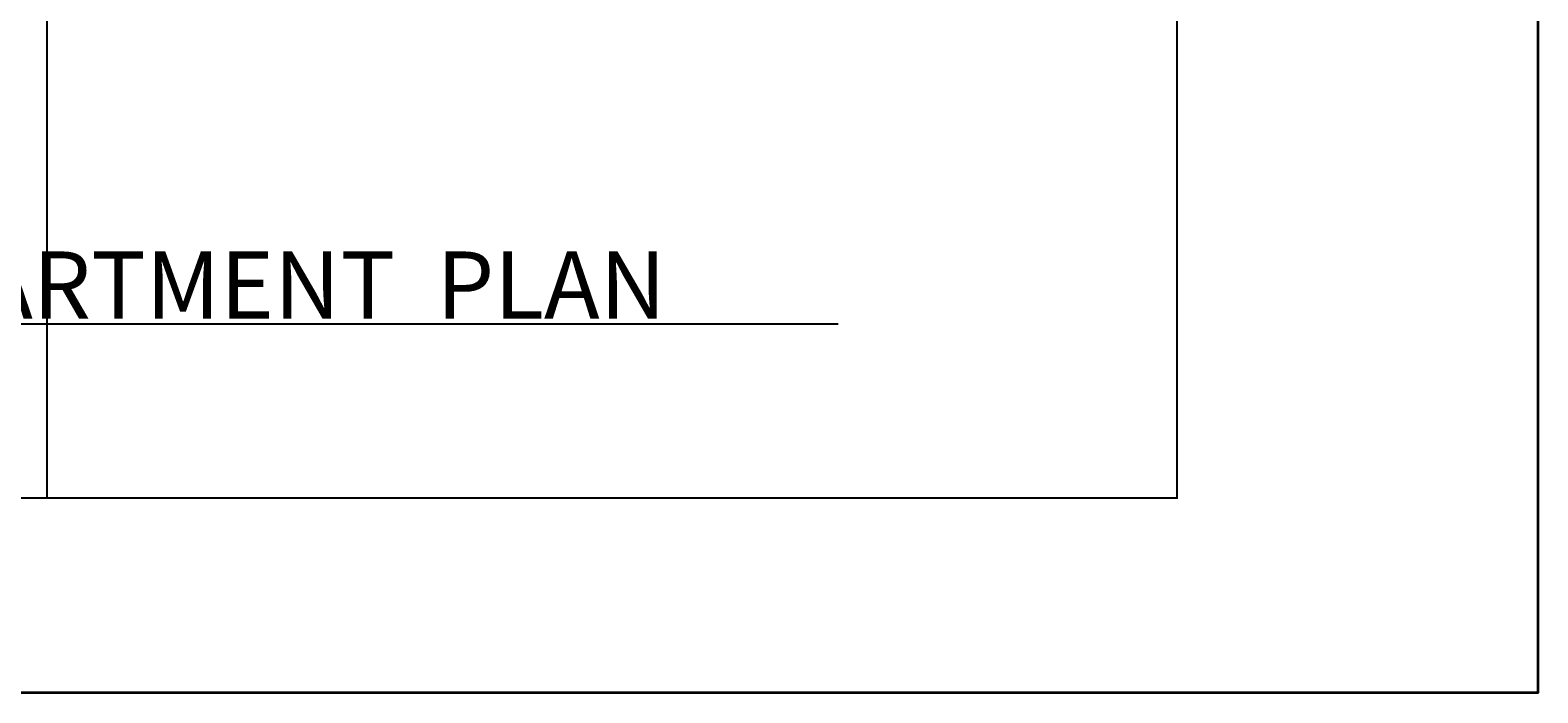
# Model space of a CAD drawing. Units: inches. Extents: x 2314 to 3223, y 1382 to 2735.
# Tile 3 of 14: x 2818 to 3223, y 1382 to 1560. Entities that reach past the tile are written whole.
import ezdxf

# ---------------------------------------------------------------- set-up
doc = ezdxf.new("R2010")
doc.units = ezdxf.units.IN
for name, color, linetype, lineweight in [('A-ANNO-DIMS', 2, 'Continuous', 18), ('A-ANNO-TEXT', 7, 'Continuous', 25), ('A-ANNO-TTLB', 7, 'Continuous', 35)]:
    doc.layers.add(name, color=color, linetype=linetype, lineweight=lineweight)
doc.layers.add('A-WALL-PATT', color=251, linetype='Continuous', lineweight=13, true_color=0x636466)
doc.styles.get("Standard").update_dxf_attribs({"font": 'arial.ttf'})
doc.dimstyles.get("Standard").update_dxf_attribs({"dimtxt": 0.18, "dimasz": 0.18, "dimexe": 0.18, "dimexo": 0.0625, "dimgap": 0.09, "dimtad": 0, "dimtih": 1, "dimtoh": 1, "dimdec": 4, "dimzin": 0, "dimdsep": 46, "dimtxsty": 'Standard', "dimcen": 0.09, "dimadec": 0, "dimazin": 0, "dimtfac": 1, "dimtdec": 4, "dimtofl": 0, "dimtmove": 0, "dimatfit": 3, "dimfxl": 1, "dimtolj": 1, "dimtzin": 0, "dimarcsym": 0})

# ---------------------------------------------------------------- blocks, each defined once
blk = doc.blocks.new('*D29')
at = {"layer": 'A-ANNO-DIMS', "color": 0, "lineweight": -2, "transparency": 16777216}
for p, q in [((2410.39, 1608.32), (2410.39, 1434.13)), ((3125.89, 1608.32), (3125.89, 1434.13)), ((2410.57, 1434.31), (2767.75, 1434.31)), ((3125.71, 1434.31), (2768.54, 1434.31))]:
    blk.add_line(p, q, dxfattribs=at)
at = {"layer": 'A-ANNO-DIMS', "color": 0, "transparency": 16777216}
for points in [[(2410.57, 1434.34), (2410.57, 1434.28), (2410.39, 1434.31)], [(3125.71, 1434.34), (3125.71, 1434.28), (3125.89, 1434.31)]]:
    blk.add_solid(points, dxfattribs=at)
at = {"layer": 'Defpoints', "color": 0, "transparency": 16777216}
for p in [(2410.39, 1608.38), (3125.89, 1608.38), (3125.89, 1434.31)]:
    blk.add_point(p, dxfattribs=at)
at = {"layer": 'A-ANNO-DIMS', "color": 0, "transparency": 16777216, "insert": (2768.14, 1434.31), "char_height": 0.18, "attachment_point": 5}
blk.add_mtext('\\A1;715.5', dxfattribs=at)
blk = doc.blocks.new('*D37')
at = {"layer": 'A-ANNO-DIMS', "color": 0, "lineweight": -2, "transparency": 16777216}
for p, q in [((2717.89, 1564.56), (2717.89, 1434.13)), ((2822.89, 1564.56), (2822.89, 1434.13)), ((2718.07, 1434.31), (2770.11, 1434.31)), ((2822.71, 1434.31), (2770.67, 1434.31))]:
    blk.add_line(p, q, dxfattribs=at)
at = {"layer": 'A-ANNO-DIMS', "color": 0, "transparency": 16777216}
for points in [[(2718.07, 1434.34), (2718.07, 1434.28), (2717.89, 1434.31)], [(2822.71, 1434.34), (2822.71, 1434.28), (2822.89, 1434.31)]]:
    blk.add_solid(points, dxfattribs=at)
at = {"layer": 'Defpoints', "color": 0, "transparency": 16777216}
for p in [(2717.89, 1564.62), (2822.89, 1564.62), (2822.89, 1434.31)]:
    blk.add_point(p, dxfattribs=at)
at = {"layer": 'A-ANNO-DIMS', "color": 0, "transparency": 16777216, "insert": (2770.39, 1434.31), "char_height": 0.18, "attachment_point": 5}
blk.add_mtext('\\A1;105', dxfattribs=at)

msp = doc.modelspace()

# ---------------------------------------------------------------- hatches: boundary and pattern name
at = {"layer": 'A-WALL-PATT'}
h = msp.add_hatch(color=256, dxfattribs=at)
h.dxf.hatch_style = 1
h.paths.add_polyline_path([(2443.3302, 2379.5332), (2443.3302, 2381.7832), (2410.3927, 2381.7832), (2410.3927, 2336.7008), (2414.8927, 2336.7008), (2414.8927, 2377.2832), (2443.3302, 2377.2832)])
h.paths.add_polyline_path([(2561.3645, 2379.5332), (2561.3645, 2381.7832), (2503.3302, 2381.7832), (2503.3302, 2377.2832), (2546.8927, 2377.2832), (2546.8927, 2245.2832), (2541.8787, 2245.2832), (2541.8787, 2240.7832), (2551.3927, 2240.7832), (2551.3927, 2377.2832), (2561.3645, 2377.2832)])
h.paths.add_polyline_path([(2656.0607, 2381.7832), (2597.3645, 2381.7832), (2597.3645, 2377.2832), (2617.3927, 2377.2832), (2617.3927, 2257.2832), (2584.2532, 2257.2832), (2584.2532, 2252.7832), (2625.8528, 2252.7832), (2625.8528, 2255.0332), (2625.8528, 2257.2832), (2621.8927, 2257.2832), (2621.8927, 2377.2832), (2656.0607, 2377.2832), (2656.0607, 2379.5332)])
h.paths.add_polyline_path([(2807.3418, 2381.7832), (2716.0607, 2381.7832), (2716.0607, 2377.2832), (2765.8927, 2377.2832), (2765.8927, 2257.2832), (2661.6935, 2257.2832), (2661.6935, 2252.7832), (2765.8927, 2252.7832), (2765.8927, 2146.2832), (2760.9259, 2146.2832), (2760.9259, 2141.8832), (2775.7119, 2141.8832), (2775.7119, 2146.2832), (2770.3927, 2146.2832), (2770.3927, 2252.7832), (2877.684, 2252.7832), (2877.684, 2255.0332), (2877.684, 2257.2832), (2770.3927, 2257.2832), (2770.3927, 2377.2832), (2807.3418, 2377.2832), (2807.3418, 2379.5332)])
h.paths.add_polyline_path([(2937.2118, 2381.7832), (2867.3418, 2381.7832), (2867.3418, 2377.2832), (2914.3927, 2377.2832), (2914.3927, 2257.2832), (2908.4124, 2257.2832), (2908.4124, 2252.7832), (2960.6432, 2252.7832), (2960.6432, 2255.0332), (2960.6432, 2257.2832), (2918.8927, 2257.2832), (2918.8927, 2377.2832), (2937.2118, 2377.2832)])
h.paths.add_polyline_path([(3022.1601, 2381.7832), (2973.2118, 2381.7832), (2973.2118, 2379.5332), (2973.2118, 2377.2832), (2984.8927, 2377.2832), (2984.8927, 2257.2832), (2980.0601, 2257.2832), (2980.0601, 2252.7832), (2984.8927, 2252.7832), (2984.8927, 2240.7832), (2995.668, 2240.7832), (2995.668, 2243.0332), (2995.668, 2245.2832), (2989.3927, 2245.2832), (2989.3927, 2377.2832), (3022.1601, 2377.2832), (3022.1601, 2379.5332)])
h.paths.add_polyline_path([(3125.8927, 2381.7832), (3082.1601, 2381.7832), (3082.1601, 2377.2832), (3121.3927, 2377.2832), (3121.3927, 2334.7388), (3125.8927, 2334.7388)])
h.paths.add_polyline_path([(3125.8927, 2274.7388), (3121.3927, 2274.7388), (3121.3927, 2245.2832), (3066.4832, 2245.2832), (3066.4832, 2240.7832), (3121.3927, 2240.7832), (3121.3927, 2232.1868), (3125.8927, 2232.1868)])
h.paths.add_polyline_path([(3125.8927, 2208.1868), (3121.3927, 2208.1868), (3121.3927, 2198.7832), (3037.3927, 2198.7832), (3037.3927, 2240.7832), (3041.2694, 2240.7832), (3041.2694, 2243.0332), (3041.2694, 2245.2832), (3026.8205, 2245.2832), (3026.8205, 2240.7832), (3032.8927, 2240.7832), (3032.8927, 2190.4022), (3037.3927, 2190.4022), (3037.3927, 2194.2832), (3121.3927, 2194.2832), (3121.3927, 2182.1835), (3125.8927, 2182.1835)])
h.paths.add_polyline_path([(3125.8927, 2158.1835), (3121.3927, 2158.1835), (3121.3927, 2146.2832), (3037.3927, 2146.2832), (3037.3927, 2169.3726), (3035.1427, 2169.3726), (3032.8927, 2169.3726), (3032.8927, 2146.2832), (2812.7301, 2146.2832), (2812.7301, 2144.0832), (2812.7301, 2141.8832), (2818.3927, 2141.8832), (2818.3927, 1970.1316), (2822.8927, 1970.1316), (2822.8927, 1978.8832), (2903.9846, 1978.8832), (2903.9846, 1981.1332), (2903.9846, 1983.3832), (2822.8927, 1983.3832), (2822.8927, 2115.3832), (2851.7162, 2115.3832), (2851.7162, 2117.6332), (2851.7162, 2119.8832), (2822.8927, 2119.8832), (2822.8927, 2141.8832), (3125.8927, 2141.8832)])
h.paths.add_polyline_path([(3125.8927, 2119.8832), (3081.193, 2119.8832), (3081.193, 2115.3832), (3121.3927, 2115.3832), (3121.3927, 2071.8188), (3125.8927, 2071.8188)], flags=17)
h.paths.add_polyline_path([(2989.3927, 2115.3832), (3021.193, 2115.3832), (3021.193, 2117.6332), (3021.193, 2119.8832), (2979.123, 2119.8832), (2979.123, 2115.3832), (2984.8927, 2115.3832), (2984.8927, 2019.3832), (2981.9225, 2019.3832), (2981.9225, 2014.8832), (2984.8927, 2014.8832), (2984.8927, 1983.3832), (2984.8927, 1978.8832), (2989.3927, 1978.8832), (2989.3927, 1983.3832)], flags=17)
h.paths.add_polyline_path([(2947.3927, 2115.3832), (2955.123, 2115.3832), (2955.123, 2117.6332), (2955.123, 2119.8832), (2911.7162, 2119.8832), (2911.7162, 2115.3832), (2942.8927, 2115.3832), (2942.8927, 1983.3832), (2936.7017, 1983.3832), (2936.7017, 1978.8832), (2947.3927, 1978.8832), (2947.3927, 1983.3832), (2947.3927, 2014.8832), (2960.7167, 2014.8832), (2960.7167, 2017.1332), (2960.7167, 2019.3832), (2947.3927, 2019.3832)], flags=17)
h.paths.add_polyline_path([(3037.3927, 1978.8832), (3041.8276, 1978.8832), (3041.8276, 1981.1332), (3041.8276, 1983.3832), (3025.477, 1983.3832), (3025.477, 1978.8832), (3032.8927, 1978.8832), (3032.8927, 1927.1259), (3035.1427, 1927.1259), (3037.3927, 1927.1259)])
h.paths.add_polyline_path([(3125.8927, 2011.8188), (3123.6427, 2011.8188), (3121.3927, 2011.8188), (3121.3927, 1983.3832), (3065, 1983.3832), (3065, 1978.8832), (3121.3927, 1978.8832), (3121.3927, 1970.5932), (3125.8927, 1970.5932)], flags=17)
h.paths.add_polyline_path([(2994.2341, 1983.3832), (2989.3927, 1983.3832), (2989.3927, 1978.8832), (2994.2341, 1978.8832), (2994.2341, 1981.1332)], flags=16)
h.paths.add_polyline_path([(3125.8927, 1946.5932), (3121.3927, 1946.5932), (3121.3927, 1936.8832), (3037.3927, 1936.8832), (3037.3927, 1932.3832), (3121.3927, 1932.3832), (3121.3927, 1919.825), (3125.8927, 1919.825)])
h.paths.add_polyline_path([(3125.8927, 1883.825), (3121.3927, 1883.825), (3121.3927, 1866.3832), (3037.3927, 1866.3832), (3037.3927, 1899.0954), (3035.1427, 1899.0954), (3032.8927, 1899.0954), (3032.8927, 1866.3832), (2822.8927, 1866.3832), (2822.8927, 1938.7212), (2820.6427, 1938.7212), (2818.3927, 1938.7212), (2818.3927, 1786.9239), (2822.8927, 1786.9239), (2822.8927, 1861.8832), (3032.8927, 1861.8832), (3032.8927, 1825.1023), (3037.3927, 1825.1023), (3037.3927, 1861.8832), (3121.3927, 1861.8832), (3121.3927, 1844.6765), (3125.8927, 1844.6765)])
h.paths.add_polyline_path([(3125.8927, 1808.6765), (3121.3927, 1808.6765), (3121.3927, 1795.8832), (3037.3927, 1795.8832), (3037.3927, 1799.4755), (3032.8927, 1799.4755), (3032.8927, 1749.3832), (3026.5034, 1749.3832), (3026.5034, 1744.8832), (3032.8927, 1744.8832), (3034.9255, 1744.8832), (3043.1326, 1744.8832), (3043.1326, 1747.1332), (3043.1326, 1749.3832), (3037.3927, 1749.3832), (3037.3927, 1791.3832), (3121.3927, 1791.3832), (3121.3927, 1783.3103), (3125.8927, 1783.3103)])
h.paths.add_polyline_path([(3125.8927, 1759.3103), (3121.3927, 1759.3103), (3121.3927, 1749.3832), (3065.1845, 1749.3832), (3065.1845, 1744.8832), (3121.3927, 1744.8832), (3121.3927, 1709.3573), (3125.8927, 1709.3573)])
h.paths.add_polyline_path([(3125.8927, 1649.3573), (3121.3927, 1649.3573), (3121.3927, 1612.8832), (3095.116, 1612.8832), (3095.116, 1608.3832), (3125.8927, 1608.3832)])
h.paths.add_polyline_path([(3035.116, 1612.8832), (2993.8927, 1612.8832), (2993.8927, 1744.8832), (2998.7409, 1744.8832), (2998.7409, 1749.3832), (2989.3927, 1749.3832), (2989.3927, 1744.8832), (2989.3927, 1701.3832), (2972.8226, 1701.3832), (2972.8226, 1696.8832), (2989.3927, 1696.8832), (2989.3927, 1612.8832), (2978.2225, 1612.8832), (2978.2225, 1608.3832), (3035.116, 1608.3832), (3035.116, 1610.6332)])
h.paths.add_polyline_path([(2947.3927, 1696.8832), (2950.7566, 1696.8832), (2950.7566, 1699.1332), (2950.7566, 1701.3832), (2947.3927, 1701.3832), (2947.3927, 1744.8832), (2947.3927, 1749.3832), (2937.649, 1749.3832), (2937.649, 1744.8832), (2942.8927, 1744.8832), (2942.8927, 1612.8832), (2907.783, 1612.8832), (2907.783, 1608.3832), (2954.2225, 1608.3832), (2954.2225, 1610.6332), (2954.2225, 1612.8832), (2947.3927, 1612.8832)])
h.paths.add_polyline_path([(2822.8927, 1744.8832), (2905.3491, 1744.8832), (2905.3491, 1747.1332), (2905.3491, 1749.3832), (2822.8927, 1749.3832), (2822.8927, 1756.9185), (2818.3927, 1756.9185), (2818.3927, 1612.8832), (2818.3927, 1569.1205), (2722.3927, 1569.1205), (2722.3927, 1612.8832), (2722.3927, 1756.9185), (2717.8927, 1756.9185), (2717.8927, 1750.0143), (2633.6297, 1750.0143), (2633.6437, 1745.2665), (2717.8927, 1745.5143), (2717.8927, 1612.8832), (2689.8467, 1612.8832), (2689.8467, 1608.3832), (2717.8927, 1608.3832), (2717.8927, 1564.6205), (2722.3927, 1564.6205), (2822.8927, 1564.6205), (2822.8927, 1569.1205), (2822.8927, 1608.3832), (2847.783, 1608.3832), (2847.783, 1610.6332), (2847.783, 1612.8832), (2822.8927, 1612.8832)])
h.paths.add_polyline_path([(2629.8467, 1612.8832), (2597.8927, 1612.8832), (2597.8927, 1744.8832), (2597.8927, 1745.1613), (2601.5887, 1745.1721), (2601.5816, 1747.5932), (2601.5745, 1750.0143), (2593.3927, 1750.0143), (2593.3927, 1744.8832), (2593.3927, 1713.3832), (2589.7588, 1713.3832), (2589.7588, 1708.8832), (2593.3927, 1708.8832), (2593.3927, 1612.8832), (2582.3793, 1612.8832), (2582.3793, 1608.3832), (2629.8467, 1608.3832), (2629.8467, 1610.6332)])
h.paths.add_polyline_path([(2551.3927, 1708.8832), (2567.6776, 1708.8832), (2567.6776, 1711.1332), (2567.6776, 1713.3832), (2551.3927, 1713.3832), (2551.3927, 1744.8832), (2551.3927, 1750.0143), (2543.5657, 1750.0143), (2543.5657, 1747.5079), (2543.5657, 1745.0014), (2546.8927, 1745.0112), (2546.8927, 1744.8832), (2546.8927, 1612.8832), (2502.9339, 1612.8832), (2502.9339, 1608.3832), (2558.3793, 1608.3832), (2558.3793, 1610.6332), (2558.3793, 1612.8832), (2551.3927, 1612.8832)])
h.paths.add_polyline_path([(2414.8927, 1656.2547), (2410.3927, 1656.2547), (2410.3927, 1608.3832), (2442.9339, 1608.3832), (2442.9339, 1610.6332), (2442.9339, 1612.8832), (2414.8927, 1612.8832)])
h.paths.add_polyline_path([(2414.8927, 1744.8832), (2468.8906, 1744.8832), (2468.8906, 1747.1332), (2468.8906, 1749.3832), (2414.8927, 1749.3832), (2414.8927, 1757.7622), (2410.3927, 1757.7622), (2410.3927, 1716.2547), (2414.8927, 1716.2547)])
h.paths.add_polyline_path([(2414.8927, 1791.3832), (2498.8927, 1791.3832), (2498.8927, 1749.3832), (2492.9799, 1749.3832), (2492.9799, 1744.8832), (2498.8927, 1744.8832), (2503.3927, 1744.8832), (2508.0135, 1744.8968), (2508.0059, 1747.4556), (2507.9984, 1750.0143), (2503.3927, 1750.0143), (2503.3927, 1802.6362), (2501.1427, 1802.6362), (2498.8927, 1802.6362), (2498.8927, 1795.8832), (2414.8927, 1795.8832), (2414.8927, 1808.0943), (2410.3927, 1808.0943), (2410.3927, 1781.7622), (2414.8927, 1781.7622)])
h.paths.add_polyline_path([(2722.3927, 1937.589), (2720.1427, 1937.589), (2717.8927, 1937.589), (2717.8927, 1866.3832), (2503.3927, 1866.3832), (2503.3927, 1896.3484), (2498.8927, 1896.3484), (2498.8927, 1866.3832), (2414.8927, 1866.3832), (2414.8927, 1882.1496), (2410.3927, 1882.1496), (2410.3927, 1844.0943), (2414.8927, 1844.0943), (2414.8927, 1861.8832), (2498.8927, 1861.8832), (2498.8927, 1831.4783), (2501.1427, 1831.4783), (2503.3927, 1831.4783), (2503.3927, 1861.8832), (2717.8927, 1861.8832), (2717.8927, 1786.9239), (2722.3927, 1786.9239)])
h.paths.add_polyline_path([(2414.8927, 1932.3832), (2498.8927, 1932.3832), (2498.8927, 1924.7883), (2503.3927, 1924.7883), (2503.3927, 1978.8832), (2505.8599, 1978.8832), (2505.8599, 1981.1332), (2505.8599, 1983.3832), (2493.3697, 1983.3832), (2493.3697, 1978.8832), (2498.8927, 1978.8832), (2498.8927, 1936.8832), (2414.8927, 1936.8832), (2414.8927, 1943.2834), (2410.3927, 1943.2834), (2410.3927, 1918.1496), (2414.8927, 1918.1496)])
h.paths.add_polyline_path([(2414.8927, 2020.3133), (2412.6427, 2020.3133), (2410.3927, 2020.3133), (2410.3927, 1967.2834), (2414.8927, 1967.2834), (2414.8927, 1978.8832), (2468.8513, 1978.8832), (2468.8513, 1981.1332), (2468.8513, 1983.3832), (2414.8927, 1983.3832)])
h.paths.add_polyline_path([(2414.8927, 2115.3832), (2453.004, 2115.3832), (2453.004, 2117.6332), (2453.004, 2119.8832), (2410.3927, 2119.8832), (2410.3927, 2080.3133), (2414.8927, 2080.3133)], flags=17)
h.paths.add_polyline_path([(2559.0969, 2117.6332), (2559.0969, 2119.8832), (2513.004, 2119.8832), (2513.004, 2115.3832), (2546.8927, 2115.3832), (2546.8927, 1983.3832), (2542.7531, 1983.3832), (2542.7531, 1978.8832), (2551.3927, 1978.8832), (2551.3927, 2014.8832), (2570.3098, 2014.8832), (2570.3098, 2017.1332), (2570.3098, 2019.3832), (2551.3927, 2019.3832), (2551.3927, 2115.3832), (2559.0969, 2115.3832)], flags=17)
h.paths.add_polyline_path([(2628.5073, 2117.6332), (2628.5073, 2119.8832), (2583.0969, 2119.8832), (2583.0969, 2115.3832), (2593.3927, 2115.3832), (2593.3927, 2019.3832), (2590.2108, 2019.3832), (2590.2108, 2014.8832), (2593.3927, 2014.8832), (2593.3927, 1978.8832), (2601.5907, 1978.8832), (2601.5907, 1981.1332), (2601.5907, 1983.3832), (2597.8927, 1983.3832), (2597.8927, 2115.3832), (2628.5073, 2115.3832)], flags=17)
h.paths.add_polyline_path([(2722.3927, 2141.8832), (2726.9871, 2141.8832), (2726.9871, 2144.2705), (2726.9871, 2146.2832), (2503.3927, 2146.2832), (2503.3927, 2168.2161), (2501.1427, 2168.2161), (2498.8927, 2168.2161), (2498.8927, 2146.2832), (2414.8927, 2146.2832), (2414.8927, 2156.5041), (2410.3927, 2156.5041), (2410.3927, 2141.8832), (2717.8927, 2141.8832), (2717.8927, 2119.8832), (2688.5073, 2119.8832), (2688.5073, 2115.3832), (2717.8927, 2115.3832), (2717.8927, 1983.3832), (2633.2454, 1983.3832), (2633.2454, 1978.8832), (2717.8927, 1978.8832), (2717.8927, 1970.1316), (2720.1427, 1970.1316), (2722.3927, 1970.1316)])
h.paths.add_polyline_path([(2557.3704, 1462.9278), (2940.0934, 1462.9278), (2940.0934, 1512.3848), (2557.3704, 1512.3848)], flags=9)
h.paths.add_polyline_path([(2846.2527, 1703.1384), (2892.8612, 1703.1384), (2892.8612, 1725.5272), (2846.2527, 1725.5272)], flags=25)
h.paths.add_polyline_path([(2885.6102, 1812.1147), (2946.1505, 1812.1147), (2946.1505, 1834.5035), (2885.6102, 1834.5035)], flags=25)
h.paths.add_polyline_path([(2885.6102, 1884.183), (2946.1505, 1884.183), (2946.1505, 1906.5718), (2885.6102, 1906.5718)], flags=25)
h.paths.add_polyline_path([(3066.365, 1705.5431), (3112.9735, 1705.5431), (3112.9735, 1727.9319), (3066.365, 1727.9319)], flags=9)
h.paths.add_polyline_path([(3061.8255, 1887.7513), (3101.6154, 1887.7513), (3101.6154, 1910.1401), (3061.8255, 1910.1401)], flags=25)
h.paths.add_polyline_path([(3063.3679, 1816.2121), (3103.1578, 1816.2121), (3103.1578, 1838.6009), (3063.3679, 1838.6009)], flags=25)
h.paths.add_polyline_path([(3053.3743, 1768.416), (3107.1329, 1768.416), (3107.1329, 1790.8048), (3053.3743, 1790.8048)], flags=25)
h.paths.add_polyline_path([(3061.6068, 1943.822), (3115.3653, 1943.822), (3115.3653, 1966.2109), (3061.6068, 1966.2109)], flags=9)
h.paths.add_polyline_path([(2745.0978, 1763.6604), (2797.9354, 1763.6604), (2797.9354, 1776.0247), (2745.0978, 1776.0247)], flags=9)
h.paths.add_polyline_path([(2574.2135, 1819.2586), (2634.7538, 1819.2586), (2634.7538, 1841.6474), (2574.2135, 1841.6474)], flags=25)
h.paths.add_polyline_path([(2574.2135, 1891.3269), (2634.7538, 1891.3269), (2634.7538, 1913.7157), (2574.2135, 1913.7157)], flags=25)
h.paths.add_polyline_path([(2638.4466, 1702.43), (2685.0551, 1702.43), (2685.0551, 1724.8188), (2638.4466, 1724.8188)], flags=25)
h.paths.add_polyline_path([(2435.9715, 1697.1215), (2482.5799, 1697.1215), (2482.5799, 1719.5103), (2435.9715, 1719.5103)], flags=9)
h.paths.add_polyline_path([(2431.2046, 1893.7833), (2470.9945, 1893.7833), (2470.9945, 1916.1721), (2431.2046, 1916.1721)], flags=25)
h.paths.add_polyline_path([(2439.8144, 1817.2116), (2479.6043, 1817.2116), (2479.6043, 1839.6004), (2439.8144, 1839.6004)], flags=25)
h.paths.add_polyline_path([(2441.2607, 1753.0942), (2495.0192, 1753.0942), (2495.0192, 1775.483), (2441.2607, 1775.483)], flags=25)
h.paths.add_polyline_path([(2421.216, 1945.3109), (2474.9746, 1945.3109), (2474.9746, 1967.6997), (2421.216, 1967.6997)], flags=25)
h.paths.add_polyline_path([(2585.4464, 1627.5703), (2585.4464, 1679), (2563.0576, 1679), (2563.0576, 1627.5703)], flags=9)
h.paths.add_polyline_path([(2978.3497, 1618.7039), (2978.3497, 1670.1337), (2955.9609, 1670.1337), (2955.9609, 1618.7039)], flags=9)
h.paths.add_polyline_path([(2975.9502, 2041.7828), (2975.9502, 2093.2125), (2953.5614, 2093.2125), (2953.5614, 2041.7828)], flags=25)
h.paths.add_polyline_path([(2835.6537, 1989.2068), (2882.2621, 1989.2068), (2882.2621, 2011.5956), (2835.6537, 2011.5956)], flags=25)
h.paths.add_polyline_path([(2649.3769, 1997.5659), (2695.9853, 1997.5659), (2695.9853, 2019.9547), (2649.3769, 2019.9547)], flags=25)
h.paths.add_polyline_path([(2579.9087, 2040.3429), (2579.9087, 2091.7726), (2557.5198, 2091.7726), (2557.5198, 2040.3429)], flags=25)
h.paths.add_polyline_path([(2783.2404, 1883.1956), (2783.2404, 2067.1369), (2764.694, 2067.1369), (2764.694, 1883.1956)], flags=9)
h.paths.add_polyline_path([(3055.8435, 1993.5571), (3102.4519, 1993.5571), (3102.4519, 2015.9459), (3055.8435, 2015.9459)], flags=25)
h.paths.add_polyline_path([(2423.6009, 1984.6082), (2470.2094, 1984.6082), (2470.2094, 2006.997), (2423.6009, 2006.997)], flags=25)
h.paths.add_polyline_path([(2973.4115, 2123.1668), (3013.1319, 2123.1668), (3013.1319, 2135.531), (2973.4115, 2135.531)], flags=25)
h.paths.add_polyline_path([(2534.3846, 2124.6231), (2574.105, 2124.6231), (2574.105, 2136.9874), (2534.3846, 2136.9874)], flags=25)
h.paths.add_polyline_path([(2829.1368, 2188.1931), (2889.411, 2188.1931), (2889.411, 2210.5819), (2829.1368, 2210.5819)], flags=9)
h.paths.add_polyline_path([(2633.2547, 2185.0437), (2693.5289, 2185.0437), (2693.5289, 2207.4325), (2633.2547, 2207.4325)], flags=9)
h.paths.add_polyline_path([(2445.1812, 2167.0395), (2496.611, 2167.0395), (2496.611, 2189.4284), (2445.1812, 2189.4284)], flags=9)
h.paths.add_polyline_path([(2429.1678, 2194.5482), (2480.5975, 2194.5482), (2480.5975, 2216.937), (2429.1678, 2216.937)], flags=9)
h.paths.add_polyline_path([(3060.1138, 2158.1056), (3111.5436, 2158.1056), (3111.5436, 2180.4944), (3060.1138, 2180.4944)], flags=9)
h.paths.add_polyline_path([(3055.6824, 2201.2631), (3107.1122, 2201.2631), (3107.1122, 2223.652), (3055.6824, 2223.652)], flags=25)
h.paths.add_polyline_path([(3044.3482, 2257.7345), (3090.9567, 2257.7345), (3090.9567, 2280.1233), (3044.3482, 2280.1233)], flags=9)
h.paths.add_polyline_path([(2942.5437, 2306.9625), (2982.3336, 2306.9625), (2982.3336, 2329.3513), (2942.5437, 2329.3513)], flags=9)
h.paths.add_polyline_path([(2799.5865, 2259.1663), (2846.195, 2259.1663), (2846.195, 2281.5551), (2799.5865, 2281.5551)], flags=25)
h.paths.add_polyline_path([(2670.4998, 2261.1493), (2717.1082, 2261.1493), (2717.1082, 2283.5381), (2670.4998, 2283.5381)], flags=25)
h.paths.add_polyline_path([(2553.0333, 2302.7735), (2592.8232, 2302.7735), (2592.8232, 2325.1624), (2553.0333, 2325.1624)], flags=9)
h.paths.add_polyline_path([(2432.0288, 2268.6489), (2478.6372, 2268.6489), (2478.6372, 2291.0377), (2432.0288, 2291.0377)], flags=9)
h = msp.add_hatch(color=256, dxfattribs=at)
h.dxf.hatch_style = 1
h.paths.add_polyline_path([(2503.3927, 2240.7832), (2507.7952, 2240.7832), (2507.7952, 2245.2832), (2496.4262, 2245.2832), (2496.4262, 2243.0332), (2496.4262, 2240.7832), (2498.8927, 2240.7832), (2498.8927, 2198.7832), (2414.8927, 2198.7832), (2414.8927, 2206.5718), (2410.3927, 2206.5718), (2410.3927, 2180.5041), (2412.6427, 2180.5041), (2414.8927, 2180.5041), (2414.8927, 2194.2832), (2498.8927, 2194.2832), (2498.8927, 2191.0069), (2503.3927, 2191.0069)])
h.paths.add_polyline_path([(2414.8927, 2276.7008), (2410.3927, 2276.7008), (2410.3927, 2230.5718), (2414.8927, 2230.5718), (2414.8927, 2240.7832), (2474.2564, 2240.7832), (2474.2564, 2243.0332), (2474.2564, 2245.2832), (2414.8927, 2245.2832)])
h.paths.add_polyline_path([(2557.3704, 1462.9278), (2940.0934, 1462.9278), (2940.0934, 1512.3848), (2557.3704, 1512.3848)], flags=9)
h.paths.add_polyline_path([(2846.2527, 1703.1384), (2892.8612, 1703.1384), (2892.8612, 1725.5272), (2846.2527, 1725.5272)], flags=9)
h.paths.add_polyline_path([(2885.6102, 1812.1147), (2946.1505, 1812.1147), (2946.1505, 1834.5035), (2885.6102, 1834.5035)], flags=9)
h.paths.add_polyline_path([(2885.6102, 1884.183), (2946.1505, 1884.183), (2946.1505, 1906.5718), (2885.6102, 1906.5718)], flags=9)
h.paths.add_polyline_path([(3066.365, 1705.5431), (3112.9735, 1705.5431), (3112.9735, 1727.9319), (3066.365, 1727.9319)], flags=9)
h.paths.add_polyline_path([(3061.8255, 1887.7513), (3101.6154, 1887.7513), (3101.6154, 1910.1401), (3061.8255, 1910.1401)], flags=9)
h.paths.add_polyline_path([(3063.3679, 1816.2121), (3103.1578, 1816.2121), (3103.1578, 1838.6009), (3063.3679, 1838.6009)], flags=9)
h.paths.add_polyline_path([(3053.3743, 1768.416), (3107.1329, 1768.416), (3107.1329, 1790.8048), (3053.3743, 1790.8048)], flags=9)
h.paths.add_polyline_path([(3061.6068, 1943.822), (3115.3653, 1943.822), (3115.3653, 1966.2109), (3061.6068, 1966.2109)], flags=9)
h.paths.add_polyline_path([(2745.0978, 1763.6604), (2797.9354, 1763.6604), (2797.9354, 1776.0247), (2745.0978, 1776.0247)], flags=9)
h.paths.add_polyline_path([(2574.2135, 1819.2586), (2634.7538, 1819.2586), (2634.7538, 1841.6474), (2574.2135, 1841.6474)], flags=9)
h.paths.add_polyline_path([(2574.2135, 1891.3269), (2634.7538, 1891.3269), (2634.7538, 1913.7157), (2574.2135, 1913.7157)], flags=9)
h.paths.add_polyline_path([(2638.4466, 1702.43), (2685.0551, 1702.43), (2685.0551, 1724.8188), (2638.4466, 1724.8188)], flags=9)
h.paths.add_polyline_path([(2435.9715, 1697.1215), (2482.5799, 1697.1215), (2482.5799, 1719.5103), (2435.9715, 1719.5103)], flags=9)
h.paths.add_polyline_path([(2431.2046, 1893.7833), (2470.9945, 1893.7833), (2470.9945, 1916.1721), (2431.2046, 1916.1721)], flags=9)
h.paths.add_polyline_path([(2439.8144, 1817.2116), (2479.6043, 1817.2116), (2479.6043, 1839.6004), (2439.8144, 1839.6004)], flags=9)
h.paths.add_polyline_path([(2441.2607, 1753.0942), (2495.0192, 1753.0942), (2495.0192, 1775.483), (2441.2607, 1775.483)], flags=9)
h.paths.add_polyline_path([(2421.216, 1945.3109), (2474.9746, 1945.3109), (2474.9746, 1967.6997), (2421.216, 1967.6997)], flags=9)
h.paths.add_polyline_path([(2585.4464, 1627.5703), (2585.4464, 1679), (2563.0576, 1679), (2563.0576, 1627.5703)], flags=9)
h.paths.add_polyline_path([(2978.3497, 1618.7039), (2978.3497, 1670.1337), (2955.9609, 1670.1337), (2955.9609, 1618.7039)], flags=9)
h.paths.add_polyline_path([(2975.9502, 2041.7828), (2975.9502, 2093.2125), (2953.5614, 2093.2125), (2953.5614, 2041.7828)], flags=9)
h.paths.add_polyline_path([(2835.6537, 1989.2068), (2882.2621, 1989.2068), (2882.2621, 2011.5956), (2835.6537, 2011.5956)], flags=9)
h.paths.add_polyline_path([(2649.3769, 1997.5659), (2695.9853, 1997.5659), (2695.9853, 2019.9547), (2649.3769, 2019.9547)], flags=9)
h.paths.add_polyline_path([(2579.9087, 2040.3429), (2579.9087, 2091.7726), (2557.5198, 2091.7726), (2557.5198, 2040.3429)], flags=9)
h.paths.add_polyline_path([(2783.2404, 1883.1956), (2783.2404, 2067.1369), (2764.694, 2067.1369), (2764.694, 1883.1956)], flags=9)
h.paths.add_polyline_path([(3055.8435, 1993.5571), (3102.4519, 1993.5571), (3102.4519, 2015.9459), (3055.8435, 2015.9459)], flags=9)
h.paths.add_polyline_path([(2423.6009, 1984.6082), (2470.2094, 1984.6082), (2470.2094, 2006.997), (2423.6009, 2006.997)], flags=9)
h.paths.add_polyline_path([(2973.4115, 2123.1668), (3013.1319, 2123.1668), (3013.1319, 2135.531), (2973.4115, 2135.531)], flags=9)
h.paths.add_polyline_path([(2534.3846, 2124.6231), (2574.105, 2124.6231), (2574.105, 2136.9874), (2534.3846, 2136.9874)], flags=9)
h.paths.add_polyline_path([(2829.1368, 2188.1931), (2889.411, 2188.1931), (2889.411, 2210.5819), (2829.1368, 2210.5819)], flags=9)
h.paths.add_polyline_path([(2633.2547, 2185.0437), (2693.5289, 2185.0437), (2693.5289, 2207.4325), (2633.2547, 2207.4325)], flags=9)
h.paths.add_polyline_path([(2445.1812, 2167.0395), (2496.611, 2167.0395), (2496.611, 2189.4284), (2445.1812, 2189.4284)], flags=9)
h.paths.add_polyline_path([(2429.1678, 2208.3022), (2480.5975, 2208.3022), (2480.5975, 2230.691), (2429.1678, 2230.691)], flags=25)
h.paths.add_polyline_path([(3060.1138, 2158.1056), (3111.5436, 2158.1056), (3111.5436, 2180.4944), (3060.1138, 2180.4944)], flags=9)
h.paths.add_polyline_path([(3055.6824, 2201.2631), (3107.1122, 2201.2631), (3107.1122, 2223.652), (3055.6824, 2223.652)], flags=9)
h.paths.add_polyline_path([(3044.3482, 2257.7345), (3090.9567, 2257.7345), (3090.9567, 2280.1233), (3044.3482, 2280.1233)], flags=9)
h.paths.add_polyline_path([(2942.5437, 2306.9625), (2982.3336, 2306.9625), (2982.3336, 2329.3513), (2942.5437, 2329.3513)], flags=9)
h.paths.add_polyline_path([(2799.5865, 2259.1663), (2846.195, 2259.1663), (2846.195, 2281.5551), (2799.5865, 2281.5551)], flags=9)
h.paths.add_polyline_path([(2670.4998, 2261.1493), (2717.1082, 2261.1493), (2717.1082, 2283.5381), (2670.4998, 2283.5381)], flags=9)
h.paths.add_polyline_path([(2553.0333, 2302.7735), (2592.8232, 2302.7735), (2592.8232, 2325.1624), (2553.0333, 2325.1624)], flags=9)
h.paths.add_polyline_path([(2432.0288, 2268.6489), (2478.6372, 2268.6489), (2478.6372, 2291.0377), (2432.0288, 2291.0377)], flags=9)

# ---------------------------------------------------------------- linework, layer by layer
at = {"layer": 'A-ANNO-TEXT'}
msp.add_line((2561.7354, 1481.0145), (3035.0613, 1481.0145), dxfattribs=at)
at = {"layer": 'A-ANNO-TTLB'}
msp.add_lwpolyline([(2314.008, 2735.417), (3222.6676, 2735.417), (3222.6676, 1382.0876), (2314.008, 1382.0876)], close=True, dxfattribs=at)

# ---------------------------------------------------------------- texts
at = {"layer": 'A-ANNO-TEXT', "insert": (2565.1548, 1500.4585), "char_height": 18, "attachment_point": 1}
msp.add_mtext_dynamic_manual_height_columns('GROUND FLOOR APPARTMENT  PLAN', width=587.546926, gutter_width=12.5, heights=[0], dxfattribs=at)

# ---------------------------------------------------------------- dimensions: what is measured, and where the dimension line sits
at = {"layer": 'A-ANNO-DIMS'}
for base, p1, p2, override, picture, middle in [((3125.8927, 1434.3145), (2410.3927, 1608.3832), (3125.8927, 1608.3832), {"dimdec": 1, "dimlfac": 1, "dimrnd": 0, "dimzin": 0, "dimdsep": 46, "dimlunit": 2}, '*D29', (2768.1427, 1434.3145)), ((2822.8927, 1434.3145), (2717.8927, 1564.6205), (2822.8927, 1564.6205), {"dimdec": 0, "dimlfac": 1, "dimrnd": 0, "dimzin": 0, "dimdsep": 46, "dimlunit": 2}, '*D37', (2770.3927, 1434.3145))]:
    dim = msp.add_linear_dim(base=base, p1=p1, p2=p2, dimstyle='Standard', override=override, dxfattribs=at)
    dim.commit()
    dim.dimension.update_dxf_attribs({"geometry": picture, "text_midpoint": middle})

doc.saveas('drawing.dxf')
